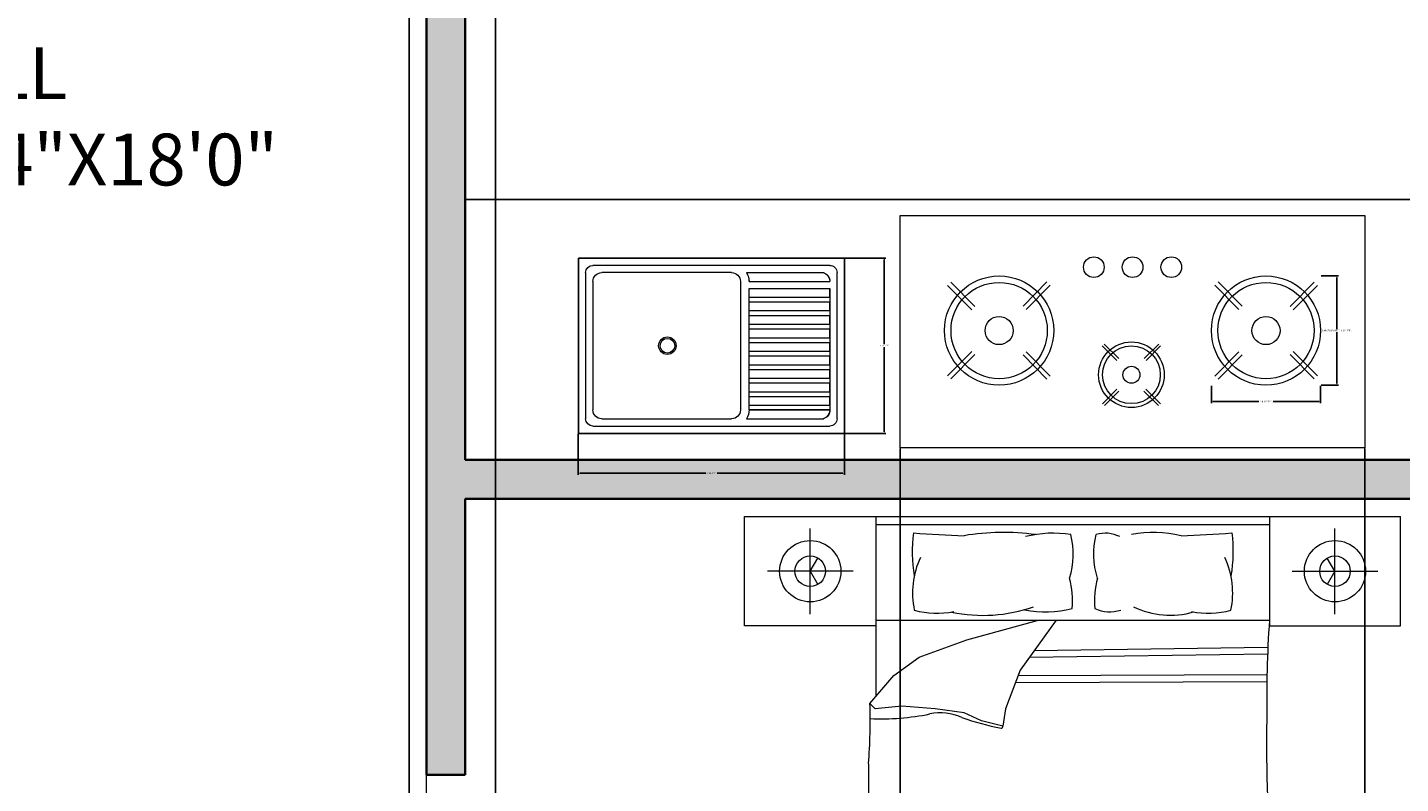
# Model space of a CAD drawing. Units: inches. Extents: x -5 to 366, y -496 to 54.
# Tile 6 of 10: x 121 to 280, y -293 to -205. Entities that reach past the tile are written whole.
import ezdxf

# ---------------------------------------------------------------- set-up
doc = ezdxf.new("R2010")
doc.units = ezdxf.units.IN
doc.header["$MEASUREMENT"] = 0
for name, color, linetype, lineweight in [('A-ANNO-DIMS', 2, 'Continuous', 18), ('A-AREA-IDEN', 7, 'Continuous', 25), ('A-DOOR', 3, 'Continuous', 18), ('A-EQPM', 9, 'Continuous', 18), ('A-FLOR-CASE', 7, 'Continuous', 25), ('A-FLOR-FIXT', 9, 'Continuous', 18), ('A-FURN', 8, 'Continuous', 18), ('A-WALL', 7, 'Continuous', 35), ('A-WALL-PATT', 252, 'Continuous', 13)]:
    doc.layers.add(name, color=color, linetype=linetype, lineweight=lineweight)
doc.styles.get("Standard").update_dxf_attribs({"font": 'arial.ttf'})
doc.dimstyles.get("Standard").update_dxf_attribs({"dimtxt": 0.18, "dimasz": 0.18, "dimexe": 0.18, "dimexo": 0.0625, "dimgap": 0.09, "dimtad": 0, "dimtih": 1, "dimtoh": 1, "dimdec": 0, "dimzin": 0, "dimdsep": 46, "dimlunit": 3, "dimtxsty": 'Standard', "dimcen": 0.09, "dimadec": 0, "dimazin": 0, "dimtfac": 1, "dimtdec": 0, "dimtofl": 0, "dimtmove": 0, "dimatfit": 3, "dimfxl": 1, "dimtolj": 1, "dimtzin": 0, "dimarcsym": 0})

# ---------------------------------------------------------------- blocks, each defined once
blk = doc.blocks.new('М12 540х820')
for p, q in [((0, 540), (-820, 540)), ((-820, 540), (-820, 0)), ((-45, 517.5), (-775, 517.5)), ((0, 0), (0, 540)), ((-797.5, 495), (-797.5, 45)), ((-775, 468), (-775, 72)), ((-347.5, 495), (-748, 495)), ((-320.5, 468), (-320.5, 72)), ((-301.7, 495), (-64.8, 495)), ((-293.7, 468), (-293.7, 472.5)), ((-293.7, 468), (-45, 468)), ((-45, 469.5), (-45, 468)), ((-22.5, 45), (-22.5, 495)), ((-293.7, 446.6), (-45, 446.6)), ((-293.7, 419.6), (-293.7, 446.6)), ((-45, 419.6), (-45, 446.6)), ((-293.7, 419.6), (-45, 419.6)), ((-293.7, 405), (-45, 405)), ((-293.7, 378), (-293.7, 405)), ((-45, 378), (-45, 405)), ((-293.7, 378), (-45, 378)), ((-293.7, 336.4), (-293.7, 363.4)), ((-293.7, 363.4), (-45, 363.4)), ((-45, 336.4), (-45, 363.4)), ((-293.7, 336.4), (-45, 336.4)), ((-293.7, 294.7), (-293.7, 321.7)), ((-293.7, 321.7), (-45, 321.7)), ((-45, 294.7), (-45, 321.7)), ((-293.7, 294.7), (-45, 294.7)), ((-293.7, 253.1), (-293.7, 280.1)), ((-293.7, 280.1), (-45, 280.1)), ((-45, 253.1), (-45, 280.1)), ((-293.7, 253.1), (-45, 253.1)), ((-293.7, 211.5), (-293.7, 238.5)), ((-293.7, 238.5), (-45, 238.5)), ((-45, 211.5), (-45, 238.5)), ((-293.7, 211.5), (-45, 211.5)), ((-293.7, 169.9), (-293.7, 196.9)), ((-293.7, 196.9), (-45, 196.9)), ((-293.7, 169.9), (-45, 169.9)), ((-45, 169.9), (-45, 196.9)), ((-293.7, 128.2), (-293.7, 155.2)), ((-293.7, 155.2), (-45, 155.2)), ((-293.7, 128.2), (-45, 128.2)), ((-45, 128.2), (-45, 155.2)), ((-293.7, 113.6), (-45, 113.6)), ((-293.7, 86.6), (-293.7, 113.6)), ((-293.7, 86.6), (-45, 86.6)), ((-45, 86.6), (-45, 113.6)), ((-748, 45), (-347.5, 45)), ((-301.7, 45), (-64.8, 45)), ((-293.7, 72), (-45, 72)), ((-45, 70.5), (-45, 72)), ((-820, 0), (0, 0)), ((-775, 22.5), (-45, 22.5))]:
    blk.add_line(p, q)
at = {"ltscale": 0.06}
for p, q in [((-820, 0), (-820, 540)), ((-820, 540), (0, 540)), ((0, 540), (0, 536.9)), ((0, 536.9), (0, 0)), ((-293.7, 446.6), (-45, 446.6)), ((-293.7, 405), (-293.7, 446.6)), ((-45, 446.6), (-45, 419.6)), ((-293.7, 363.4), (-293.7, 405)), ((-45, 419.6), (-45, 378)), ((-293.7, 321.7), (-293.7, 363.4)), ((-45, 378), (-45, 336.4)), ((-293.7, 280.1), (-293.7, 321.7)), ((-45, 336.4), (-45, 294.7)), ((-293.7, 238.5), (-293.7, 280.1)), ((-45, 294.7), (-45, 253.1)), ((-293.7, 196.9), (-293.7, 238.5)), ((-45, 253.1), (-45, 211.5)), ((-293.7, 155.2), (-293.7, 196.9)), ((-45, 211.5), (-45, 169.9)), ((-45, 169.9), (-45, 128.2)), ((-293.7, 113.6), (-293.7, 155.2)), ((-45, 128.2), (-45, 86.6)), ((-293.7, 72), (-293.7, 113.6)), ((-45, 86.6), (-45, 72)), ((-45, 72), (-293.7, 72)), ((0, 0), (-820, 0))]:
    blk.add_line(p, q, dxfattribs=at)
at = {"extrusion": (0, 0, -1)}
for centre, major_axis, start_param, end_param in [((-775, 495), (-15.9, 15.9), -0.785398, 0.785398), ((-775, 495), (-15.9, 15.9), -0.785398, 0.785398), ((-45, 495), (-15.9, -15.9), 2.356194, 3.926991), ((-45, 495), (-15.9, -15.9), 2.356194, 3.926991), ((-748, 468), (-19.1, -19.1), 0.785398, 2.356194), ((-748, 468), (-19.1, -19.1), 0.785398, 2.356194), ((-347.5, 468), (-19.1, 19.1), 0.785398, 2.356194), ((-347.5, 468), (-19.1, 19.1), 0.785398, 2.356194), ((-343.2, 468), (-35, 35), 1.779263, 2.356194), ((-343.2, 468), (-35, 35), 1.779263, 2.356192), ((-343.2, 468), (-35, 35), 2.356192, 2.356194), ((-72.3, 468.8), (-19.3, 19.3), 1.0328, 2.38382), ((-72.3, 468.8), (-19.3, 19.3), 1.0328, 1.064673), ((-72.3, 468.8), (-19.3, 19.3), 1.064673, 2.328569), ((-72.3, 468.8), (-19.3, 19.3), 2.328569, 2.38382), ((-545.5, 270), (-19.1, -19.1), 3.926991, 10.210176), ((-545.5, 270), (-19.1, -19.1), 3.926991, 10.210176), ((-545.5, 270), (-15.9, -15.9), 3.926991, 10.210176), ((-545.5, 270), (-15.9, -15.9), 3.926991, 10.210176), ((-775, 45), (-15.9, -15.9), 5.497787, 7.068583), ((-775, 45), (-15.9, -15.9), 5.497787, 7.068583), ((-748, 72), (-19.1, 19.1), 3.926991, 5.497787), ((-748, 72), (-19.1, 19.1), 3.926991, 5.497787), ((-347.5, 72), (-19.1, -19.1), 3.926991, 5.497787), ((-347.5, 72), (-19.1, -19.1), 3.926991, 5.497787), ((-343.2, 72), (-35, -35), 3.926991, 4.503922), ((-343.2, 72), (-35, -35), 3.926991, 4.503922), ((-72.3, 71.2), (-19.3, -19.3), 3.899365, 5.250385), ((-72.3, 71.2), (-19.3, -19.3), 5.218512, 5.250385), ((-72.3, 71.2), (-19.3, -19.3), 3.954617, 5.218512), ((-72.3, 71.2), (-19.3, -19.3), 3.899365, 3.954617), ((-45, 45), (-15.9, 15.9), 2.356194, 3.926991), ((-45, 45), (-15.9, 15.9), 2.356194, 3.926991)]:
    blk.add_ellipse(centre, major_axis=major_axis, ratio=1, start_param=start_param, end_param=end_param, dxfattribs=at)
blk = doc.blocks.new('BED-DOUBLE-WITH-NIGHTSTANDS')
for p, q in [((0, 64.67), (76.05, 64.67)), ((15.21, 64.67), (15.21, 43.8)), ((60.84, 63.7), (15.21, 63.7)), ((7.61, 53.37), (7.61, 63.31)), ((68.45, 53.37), (68.45, 63.31)), ((12.58, 58.34), (2.64, 58.34)), ((63.48, 58.34), (73.42, 58.34)), ((15.21, 52.66), (60.84, 52.66)), ((25.78, 50.4), (34.07, 52.66)), ((36.11, 52.66), (31.94, 46.86)), ((20.23, 48.39), (25.78, 50.4)), ((60.64, 49.5), (33.56, 49.12)), ((17.3, 46.24), (20.23, 48.39)), ((60.61, 48.72), (33, 48.33)), ((14.53, 43.01), (17.3, 46.24)), ((31.94, 46.86), (30.24, 42.39)), ((60.57, 46.32), (31.69, 46.21)), ((60.58, 45.54), (31.39, 45.42)), ((15.15, 42.39), (14.53, 43.01)), ((18.23, 42.7), (15.15, 42.39)), ((22.08, 42.39), (18.23, 42.7)), ((25.47, 41.93), (22.08, 42.39)), ((27.47, 41.01), (25.47, 41.93)), ((30.24, 42.39), (29.94, 40.39)), ((29.94, 40.39), (27.47, 41.01)), ((10.04, 27.39), (14.34, 27.39)), ((10.04, 0), (10.04, 27.39)), ((61.27, 27.39), (65.49, 27.39)), ((65.49, 27.39), (65.49, 0)), ((14.34, 26.51), (10.92, 26.51)), ((10.92, 26.51), (10.92, 0.88)), ((64.6, 26.51), (61.25, 26.51)), ((64.6, 0.88), (64.6, 26.51)), ((61.19, 22.65), (14.34, 22.65)), ((61.26, 21.7), (14.34, 21.7)), ((53.47, 14.23), (22.59, 14.23)), ((18.42, 8.59), (18.25, 9.45)), ((23.73, 8.59), (23.9, 9.45)), ((51.79, 8.59), (51.63, 9.45)), ((57.11, 8.59), (57.28, 9.45)), ((10.92, 0.88), (64.6, 0.88)), ((65.49, 0), (10.04, 0))]:
    blk.add_line(p, q)
for points in [[(15.21, 52), (0, 52), (0, 64.67)], [(60.84, 64.67), (60.84, 52), (76.05, 52), (76.05, 64.67)], [(7.61, 58.34), (8.49, 59.87)], [(68.45, 58.34), (67.56, 59.87)], [(7.61, 58.34), (8.49, 56.8)], [(68.45, 58.34), (67.56, 56.8)]]:
    blk.add_lwpolyline(points)
for points in [[(19.58, 62.78, 0.074897), (19.67, 57.81, -0.472817)], [(37.67, 57.53, 0.14099), (37.82, 62.6, 0.235245)], [(40.92, 57.53, -0.14099), (40.77, 62.6, -0.235245)], [(56.48, 62.78, -0.074897), (56.38, 57.81, 0.472817)], [(14.37, 36.04, 0.001242), (14.34, 21.61, -0.127202), (12.81, 14.42)], [(61.17, 23.25, 0.056112), (61.72, 19.07, 0.095341), (62.79, 15.03)]]:
    blk.add_lwpolyline(points, format="xyb")
for centre, radius in [((7.61, 58.34), 3.55), ((68.45, 58.34), 3.55), ((7.61, 58.34), 1.77), ((68.45, 58.34), 1.77), ((22.81, 5.83), 0.194), ((52.72, 5.83), 0.194), ((21.54, 3.79), 0.194), ((53.98, 3.79), 0.194)]:
    blk.add_circle(centre, radius)
for centre, radius, start, end in [((61.5, 786.54), 724.98, 266.68521, 267.14978), ((30, 35.26), 27.58, 82.2196, 99.497), ((35.83, 49.2), 13.55, 81.5249, 103.96), ((41.81, 58.99), 3.76, 63.3437, 106.1026), ((47.45, 49.47), 13.37, 76.3427, 101.1841), ((14.56, 786.54), 724.98, 272.85022, 273.31479), ((29.27, 55.82), 9.8, 155.1316, 191.7583), ((46.79, 55.82), 9.8, 348.2417, 24.8684), ((28.71, 54.99), 9.32, 354.0129, 15.8293), ((49.88, 54.99), 9.32, 164.1707, 185.9871), ((27.66, 70.91), 17.68, 258.0397, 289.2615), ((49.36, 62.92), 9.68, 243.8761, 286.1746), ((22.29, 63.67), 10.19, 255.1039, 281.0369), ((34.82, 67.05), 13.41, 259.8617, 283.6238), ((42.32, 57.67), 4.03, 245.0183, 288.5407), ((53.76, 63.67), 10.19, 258.9631, 284.8961), ((197.18, 43.36), 136.65, 176.1, 180.9282), ((-55.2, 41.12), 69.76, 355.8294, 1.553), ((15.83, 69.94), 28.7, 267.4519, 281.3392), ((22.69, 35.73), 6.19, 66.2616, 101.3392), ((35.22, 69.13), 29.49, 250.1194, 259.3383), ((29.76, 40.33), 0.184, 268.8623, 19.7536), ((238.78, 38.39), 178.26, 179.1145, 184.8735), ((13.51, 14.47), 0.702, 183.98, 297.3412), ((62.21, 14.65), 0.693, 246.5219, 33.8264), ((21.68, -64.93), 79.17, 89.3433, 95.6887), ((16.57, 11.64), 1.28, 84.4856, 181.0538), ((13.22, 8.88), 5.76, 33.6671, 63.2997), ((16.17, 10.69), 2.29, 355.2933, 76.921), ((20.93, 12.3), 2.93, 145.785, 184.7304), ((15.33, 13.67), 3.15, 328.8218, 9.1554), ((19.23, 13.39), 0.916, 120.0293, 142.325), ((17.77, 12.85), 2.42, 289.2822, 29.1751), ((17.4, 12.41), 2.19, 7.436, 29.9149), ((18.84, 13.57), 1.14, 311.5653, 23.8354), ((19.23, 13.39), 0.916, 44.4517, 63.558), ((24.38, 12.85), 2.42, 150.8249, 250.7178), ((23.31, 13.57), 1.14, 156.1646, 228.4347), ((22.92, 13.39), 0.916, 113.229, 135.5483), ((24.75, 12.41), 2.19, 150.0851, 172.564), ((22.92, 13.39), 0.916, 37.675, 66.7144), ((21.22, 12.3), 2.93, 355.2696, 34.215), ((26.82, 13.67), 3.15, 169.7133, 211.1782), ((25.97, 10.69), 2.29, 103.079, 184.7067), ((28.93, 8.88), 5.76, 111.4941, 146.3329), ((25.58, 11.64), 1.28, 358.9462, 95.5144), ((49.95, 11.64), 1.28, 84.4856, 181.0538), ((46.59, 8.88), 5.76, 33.6671, 68.5059), ((49.55, 10.69), 2.29, 355.2933, 76.921), ((54.31, 12.3), 2.93, 145.785, 184.7304), ((48.7, 13.67), 3.15, 328.8218, 10.2867), ((52.61, 13.39), 0.916, 113.2856, 142.325), ((51.15, 12.85), 2.42, 289.2822, 29.1751), ((50.78, 12.41), 2.19, 7.436, 29.9149), ((52.61, 13.39), 0.916, 44.4517, 66.7144), ((52.22, 13.57), 1.14, 311.5653, 23.8354), ((55.8, -59.74), 74, 85.2402, 91.8035), ((57.76, 12.85), 2.42, 150.8249, 250.7178), ((56.68, 13.57), 1.14, 156.1646, 228.4347), ((56.3, 13.39), 0.916, 106.6343, 135.5483), ((58.13, 12.41), 2.19, 150.0851, 172.564), ((56.3, 13.39), 0.916, 37.675, 72.5814), ((54.6, 12.3), 2.93, 355.2696, 34.215), ((60.2, 13.67), 3.15, 169.249, 211.1782), ((59.35, 10.69), 2.29, 103.079, 184.7067), ((62.31, 8.88), 5.76, 113.6453, 146.3329), ((58.96, 11.64), 1.28, 358.9462, 95.5144), ((17.09, 11.46), 1.82, 174.9449, 262.8857), ((17.81, 12.15), 1.76, 201.5819, 291.4221), ((17.47, 10.23), 1.89, 299.9085, 73.1337), ((18.67, 11.02), 0.472, 257.3041, 15.1471), ((20.63, 11.55), 1.56, 131.5653, 195.1471), ((21.52, 11.55), 1.56, 344.8529, 48.4347), ((24.67, 10.23), 1.89, 106.8663, 240.0915), ((23.48, 11.02), 0.472, 164.8529, 282.6959), ((24.34, 12.15), 1.76, 248.5779, 338.4181), ((25.05, 11.46), 1.82, 277.1143, 5.0551), ((50.47, 11.46), 1.82, 174.9449, 262.8857), ((51.19, 12.15), 1.76, 201.5819, 291.4221), ((50.85, 10.23), 1.89, 299.9085, 73.1337), ((52.05, 11.02), 0.472, 257.3041, 15.1471), ((54.01, 11.55), 1.56, 131.5653, 195.1471), ((54.89, 11.55), 1.56, 344.8529, 48.4347), ((58.05, 10.23), 1.89, 106.8663, 240.0915), ((56.86, 11.02), 0.472, 164.8529, 282.6959), ((57.72, 12.15), 1.76, 248.5779, 338.4181), ((58.43, 11.46), 1.82, 277.1143, 5.0551), ((16.68, 8.53), 1.14, 80.264, 250.8688), ((14.41, 11.04), 3.59, 301.2614, 341.7045), ((16.78, 11.86), 2.21, 272.3591, 324.0401), ((14.38, 10.75), 4.08, 326.2883, 356.5076), ((20.93, 12.3), 2.93, 212.7011, 216.3445), ((21.29, 10.31), 0.147, 102.7051, 280.4384), ((21.28, 10.4), 0.238, 280.4384, 100.4136), ((21.22, 12.3), 2.93, 323.6555, 327.2989), ((25.37, 11.86), 2.21, 215.9599, 267.6409), ((27.77, 10.75), 4.08, 183.4924, 213.7117), ((27.73, 11.04), 3.59, 198.2955, 238.7386), ((25.47, 8.53), 1.14, 289.1312, 99.736), ((38.64, 9.21), 0.823, 63.0274, 163.8037), ((37.8, 11.14), 1.7, 271.4585, 315.3727), ((38.49, 8.01), 1.57, 45.5411, 114.3101), ((39.57, 8.01), 1.57, 65.6899, 134.4589), ((39.42, 9.21), 0.823, 16.1963, 116.9726), ((40.26, 11.14), 1.7, 224.6273, 268.5415), ((50.06, 8.53), 1.14, 80.264, 250.8688), ((47.79, 11.04), 3.59, 301.2614, 341.7045), ((50.16, 11.86), 2.21, 272.3591, 324.0401), ((47.76, 10.75), 4.08, 326.2883, 356.5076), ((54.31, 12.3), 2.93, 212.7011, 216.3445), ((54.25, 10.4), 0.238, 79.5864, 259.5616), ((54.23, 10.31), 0.147, 259.5616, 77.2949), ((54.6, 12.3), 2.93, 323.6555, 327.2989), ((58.75, 11.86), 2.21, 215.9599, 267.6409), ((61.15, 10.75), 4.08, 183.4924, 213.7117), ((61.11, 11.04), 3.59, 198.2955, 238.7386), ((58.85, 8.53), 1.14, 289.1312, 99.736), ((16.44, 7.29), 0.7, 63.9755, 143.2681), ((16.4, 8.87), 1.43, 265.969, 344.3045), ((17.94, 6.98), 1.52, 96.1662, 141.5825), ((20.45, 8.04), 0.399, 101.3256, 154.4621), ((19.88, 9.4), 1.2, 280.2588, 300.656), ((20.15, 10.36), 2.14, 268.3264, 277.1302), ((26.56, 6.48), 6.3, 163.5842, 183.8277), ((19.62, 9.39), 1.22, 308.2101, 316.3071), ((20.37, 8.59), 0.365, 278.3432, 4.2869), ((20.17, 8.91), 0.637, 300.656, 332.6341), ((20.64, 8.49), 0.155, 55.7657, 157.4417), ((26.56, 6.48), 6.3, 153.0032, 159.8941), ((20.89, 8.63), 0.155, 84.3784, 186.0543), ((20.74, 9.25), 0.637, 269.1859, 301.164), ((20.93, 8.93), 0.365, 237.5332, 323.4768), ((20.57, 9.97), 1.22, 285.5129, 293.6099), ((21.37, 8.59), 0.399, 87.3579, 140.4944), ((20.45, 9.74), 1.2, 301.164, 321.5612), ((19.47, 9.95), 2.14, 324.6898, 333.4936), ((24.21, 6.98), 1.52, 38.4175, 83.8338), ((25.74, 8.87), 1.43, 195.6955, 274.031), ((25.71, 7.29), 0.7, 36.7319, 116.0245), ((38.62, -0.46), 9.93, 94.4623, 172.255), ((38.66, 8.7), 1.1, 137.7873, 219.1145), ((37.41, 8.74), 0.829, 298.5391, 58.3627), ((39.93, 16.07), 6.95, 252.593, 267.2582), ((38.66, 9.41), 0.812, 177.7585, 283.852), ((40.22, 10.26), 2.51, 198.9159, 238.011), ((38.14, 16.07), 6.95, 272.7418, 287.407), ((38.83, 8.73), 0.107, 283.852, 219.9245), ((38.96, 8.23), 0.123, 238.011, 71.5592), ((38.98, 8.29), 0.0599, 71.5592, 188.0167), ((39.1, 8.23), 0.123, 108.4408, 301.989), ((39.08, 8.29), 0.0599, 351.9833, 108.4408), ((39.22, 8.77), 0.0647, 320.1909, 256.0209), ((37.84, 10.26), 2.51, 301.989, 341.0841), ((39.4, 9.41), 0.812, 256.148, 2.2415), ((40.65, 8.74), 0.829, 121.6373, 241.4609), ((39.4, 8.7), 1.1, 320.8855, 42.2127), ((39.12, 1.83), 7.69, 352.8636, 81.8197), ((49.82, 7.29), 0.7, 63.9755, 143.2681), ((49.78, 8.87), 1.43, 265.969, 344.3045), ((51.32, 6.98), 1.52, 96.1662, 141.5825), ((55.08, 9.74), 1.2, 218.4388, 238.836), ((54.15, 8.59), 0.399, 39.5056, 92.6421), ((56.06, 9.95), 2.14, 206.5064, 215.3102), ((54.6, 8.93), 0.365, 216.5232, 302.4668), ((54.95, 9.97), 1.22, 246.3901, 254.4871), ((54.79, 9.25), 0.637, 238.836, 270.8141), ((48.96, 6.48), 6.3, 20.1059, 26.9968), ((54.64, 8.63), 0.155, 353.9457, 95.6216), ((54.88, 8.49), 0.155, 22.5583, 124.2343), ((55.16, 8.59), 0.365, 175.7131, 261.6568), ((55.36, 8.91), 0.637, 207.3659, 239.344), ((48.96, 6.48), 6.3, 356.1723, 16.4158), ((55.91, 9.39), 1.22, 223.6929, 231.7899), ((55.65, 9.4), 1.2, 239.344, 259.7412), ((55.37, 10.36), 2.14, 262.8698, 271.6736), ((55.07, 8.04), 0.399, 25.5379, 78.6744), ((59.12, 8.87), 1.43, 195.6955, 274.031), ((57.59, 6.98), 1.52, 38.4175, 83.8338), ((59.08, 7.29), 0.7, 36.7319, 116.0245), ((20.52, -1.44), 9.93, 124.3865, 158.5908), ((15.99, 6.52), 1.1, 167.7115, 249.0387), ((15.71, 6.95), 0.823, 92.9516, 193.728), ((14.03, 8.2), 1.7, 301.3827, 345.2969), ((16.18, 5.84), 1.57, 75.4653, 144.2343), ((13.4, 13.54), 6.95, 282.5173, 297.1824), ((14.89, 5.93), 0.829, 328.4633, 88.2869), ((16.56, 8.65), 2.51, 228.8402, 267.9352), ((15.63, 7.13), 0.812, 207.6827, 313.7762), ((16.12, 6.62), 0.107, 313.7762, 249.7183), ((16.46, 6.32), 0.0599, 101.4834, 217.9409), ((16.48, 6.26), 0.123, 267.9352, 101.4834), ((19.32, 7.28), 0.323, 101.5637, 142.6358), ((19.06, 6.98), 0.194, 273.2768, 86.7232), ((19.32, 6.63), 0.32, 217.7621, 259.0403), ((19.28, 7.17), 0.185, 91.1081, 181.8675), ((19.66, 7.05), 0.588, 203.4276, 227.6104), ((19.48, 6.8), 0.4, 80.3487, 133.6538), ((19.41, 7.13), 0.317, 229.7889, 317.6792), ((19.06, 7.54), 0.466, 288.7263, 352.5032), ((19.05, 6.46), 0.45, 355.053, 68.3618), ((19.4, 6.38), 0.634, 83.0852, 105.7171), ((19.38, 7.52), 0.15, 345.2356, 144.9248), ((19.35, 6.43), 0.149, 232.4737, 355.053), ((15.01, 1.12), 7.22, 43.1541, 52.0459), ((19.52, 7.03), 0.167, 317.6792, 80.3487), ((21.33, 6.12), 0.883, 304.5369, 16.3699), ((22.55, 5.87), 0.625, 127.3105, 187.9252), ((21.7, 5.94), 0.641, 355.0106, 41.658), ((23.08, 6.13), 0.323, 101.5637, 176.365), ((23.14, 6.36), 0.15, 345.2356, 144.9248), ((25.67, 6.26), 0.123, 78.5166, 272.0648), ((25.96, 5.84), 1.57, 35.7657, 104.5347), ((28.74, 13.54), 6.95, 242.8176, 257.4827), ((25.58, 8.65), 2.51, 272.0648, 311.1598), ((25.68, 6.32), 0.0599, 322.0591, 78.5166), ((26.52, 7.13), 0.812, 226.2238, 332.3173), ((26.04, 6.66), 0.0647, 290.2667, 226.2271), ((27.26, 5.93), 0.829, 91.7131, 211.5367), ((26.44, 6.95), 0.823, 346.272, 87.0484), ((28.12, 8.2), 1.7, 194.7031, 238.6173), ((26.16, 6.52), 1.1, 290.9613, 12.2885), ((21.63, -1.44), 9.93, 21.4092, 55.6135), ((53.9, -1.44), 9.93, 124.3865, 158.5908), ((49.36, 6.52), 1.1, 167.7115, 249.0387), ((49.09, 6.95), 0.823, 92.9516, 193.728), ((47.41, 8.2), 1.7, 301.3827, 345.2969), ((49.56, 5.84), 1.57, 75.4653, 144.2343), ((46.78, 13.54), 6.95, 282.5173, 297.1824), ((49.01, 7.13), 0.812, 207.6827, 313.7762), ((49.94, 8.65), 2.51, 228.8402, 267.9352), ((48.26, 5.93), 0.829, 328.4633, 88.2869), ((49.5, 6.62), 0.107, 313.7762, 249.7183), ((49.84, 6.32), 0.0599, 101.4834, 217.9409), ((49.86, 6.26), 0.123, 267.9352, 101.4834), ((52.39, 6.36), 0.15, 35.0752, 194.7644), ((52.45, 6.13), 0.323, 3.635, 78.4363), ((53.83, 5.94), 0.641, 138.342, 184.9894), ((54.2, 6.12), 0.883, 163.6301, 235.4631), ((52.97, 5.87), 0.625, 352.0748, 52.6895), ((60.52, 1.12), 7.22, 127.9541, 136.8459), ((56.01, 7.03), 0.167, 99.6513, 222.3208), ((56.12, 7.13), 0.317, 222.3208, 310.2111), ((56.05, 6.8), 0.4, 46.3462, 99.6513), ((56.15, 7.52), 0.15, 35.0752, 194.7644), ((56.46, 7.54), 0.466, 187.4968, 251.2737), ((56.48, 6.46), 0.45, 111.6382, 184.947), ((56.18, 6.43), 0.149, 184.947, 307.5263), ((56.12, 6.38), 0.634, 74.2829, 96.9148), ((56.25, 7.17), 0.185, 358.1325, 88.8919), ((55.86, 7.05), 0.588, 312.3896, 336.5724), ((56.2, 7.28), 0.323, 37.3642, 78.4363), ((56.21, 6.63), 0.32, 280.9597, 322.2379), ((56.47, 6.98), 0.194, 93.2768, 266.7232), ((59.05, 6.26), 0.123, 78.5166, 272.0648), ((59.34, 5.84), 1.57, 35.7657, 104.5347), ((62.12, 13.54), 6.95, 242.8176, 257.4827), ((58.96, 8.65), 2.51, 272.0648, 311.1598), ((59.06, 6.32), 0.0599, 322.0591, 78.5166), ((59.9, 7.13), 0.812, 226.2238, 332.3173), ((59.42, 6.66), 0.0647, 290.2667, 226.2271), ((60.64, 5.93), 0.829, 91.7131, 211.5367), ((61.5, 8.2), 1.7, 194.7031, 238.6173), ((59.82, 6.95), 0.823, 346.272, 87.0484), ((59.54, 6.52), 1.1, 290.9613, 12.2885), ((55.01, -1.44), 9.93, 21.4092, 55.6135), ((3.53, -0.46), 9.93, 7.745, 41.8856), ((20, 5.48), 0.399, 101.3256, 154.4621), ((19.42, 6.84), 1.2, 280.2588, 300.656), ((19.7, 7.8), 2.14, 268.3264, 277.1302), ((19.17, 6.83), 1.22, 308.2101, 316.3071), ((20.13, 4.78), 0.216, 146.8636, 236.9021), ((23.18, 9.55), 5.66, 235.1882, 238.8844), ((20.5, 5.1), 0.585, 199.4799, 267.6828), ((19.91, 6.03), 0.365, 278.3432, 4.2869), ((19.71, 6.35), 0.637, 300.656, 332.6341), ((20.19, 5.93), 0.155, 55.7657, 157.4417), ((23.43, 6.32), 3.16, 184.756, 209.2041), ((27.97, 13.04), 10.39, 222.2412, 232.1744), ((20.65, 4.61), 0.169, 311.8703, 134.2646), ((21.14, 5.38), 0.883, 247.2305, 319.0635), ((23.75, 2.13), 3.79, 120.544, 139.818), ((21.59, 4.21), 0.625, 70.0041, 130.6188), ((21.19, 4.97), 0.641, 297.7043, 344.3516), ((21.8, 5.92), 0.537, 272.8499, 356.1226), ((21.42, 5.72), 0.52, 321.7607, 7.9252), ((21.53, 4.97), 0.52, 8.7227, 54.8872), ((21.56, 4.55), 0.883, 0.278, 72.111), ((21.95, 4.88), 0.537, 20.5253, 88.5375), ((22.66, 5.14), 0.625, 188.7227, 249.3375), ((22.4, 5.47), 0.192, 148.0499, 225.6268), ((23.75, 2.13), 3.79, 113.0501, 113.8477), ((22.76, 5.25), 0.611, 104.7558, 148.0499), ((22.42, 5.69), 0.382, 247.4086, 351.4386), ((22.6, 6.1), 0.264, 126.1046, 271.4281), ((22.57, 6.17), 0.19, 353.7526, 131.7054), ((21.86, 4.83), 0.641, 334.9899, 21.6373), ((22.52, 5.67), 0.128, 262.906, 7.132), ((22.39, 5.95), 0.267, 0.0645, 61.1507), ((22.45, 6.18), 0.305, 311.8413, 355.7877), ((23.07, 5.47), 0.32, 151.2196, 259.0403), ((23.04, 6.02), 0.185, 91.1081, 181.8675), ((23.42, 5.9), 0.588, 203.4276, 227.6104), ((23.23, 5.64), 0.4, 80.3487, 133.6538), ((23.16, 5.98), 0.317, 229.7889, 317.6792), ((22.82, 6.39), 0.466, 288.7263, 352.5032), ((22.8, 5.3), 0.45, 355.053, 68.3618), ((23.16, 5.23), 0.634, 83.0852, 105.7171), ((23.1, 5.28), 0.149, 232.4737, 355.053), ((23.27, 5.87), 0.167, 317.6792, 80.3487), ((23.75, 2.13), 3.79, 87.1071, 94.7585), ((51.78, 2.13), 3.79, 85.2415, 92.8929), ((52.25, 5.87), 0.167, 99.6513, 222.3208), ((52.37, 5.98), 0.317, 222.3208, 310.2111), ((52.29, 5.64), 0.4, 46.3462, 99.6513), ((52.71, 6.39), 0.466, 187.4968, 251.2737), ((52.72, 5.3), 0.45, 111.6382, 184.947), ((52.42, 5.28), 0.149, 184.947, 307.5263), ((52.37, 5.23), 0.634, 74.2829, 96.9148), ((52.49, 6.02), 0.185, 358.1325, 88.8919), ((52.11, 5.9), 0.588, 312.3896, 336.5724), ((52.45, 5.47), 0.32, 280.9597, 28.7804), ((53.11, 5.69), 0.382, 188.5614, 292.5914), ((52.96, 6.17), 0.19, 48.2946, 186.2474), ((53.07, 6.18), 0.305, 184.2123, 228.1587), ((53.14, 5.95), 0.267, 118.8493, 179.9355), ((53, 5.67), 0.128, 172.868, 277.094), ((52.93, 6.1), 0.264, 268.5719, 53.8954), ((52.77, 5.25), 0.611, 31.9501, 75.2442), ((53.67, 4.83), 0.641, 158.3627, 205.0101), ((53.57, 4.88), 0.537, 91.4625, 159.4747), ((53.97, 4.55), 0.883, 107.889, 179.722), ((52.87, 5.14), 0.625, 290.6625, 351.2773), ((53.73, 5.92), 0.537, 183.8774, 267.1501), ((51.78, 2.13), 3.79, 66.1523, 66.9499), ((53.12, 5.47), 0.192, 314.3732, 31.9501), ((54, 4.97), 0.52, 125.1128, 171.2773), ((54.11, 5.72), 0.52, 172.0748, 218.2393), ((51.78, 2.13), 3.79, 40.182, 59.456), ((53.93, 4.21), 0.625, 49.3812, 109.9959), ((54.39, 5.38), 0.883, 220.9365, 292.7695), ((54.34, 4.97), 0.641, 195.6484, 242.2957), ((47.55, 13.04), 10.39, 307.8256, 317.7588), ((54.88, 4.61), 0.169, 45.7354, 228.1297), ((52.1, 6.32), 3.16, 330.7959, 355.244), ((55.02, 5.1), 0.585, 272.3172, 340.5201), ((55.33, 5.93), 0.155, 22.5583, 124.2343), ((55.61, 6.03), 0.365, 175.7131, 261.6568), ((55.81, 6.35), 0.637, 207.3659, 239.344), ((52.34, 9.55), 5.66, 301.1156, 304.8118), ((56.36, 6.83), 1.22, 223.6929, 231.7899), ((56.1, 6.84), 1.2, 239.344, 259.7412), ((55.39, 4.78), 0.216, 303.0979, 33.1364), ((55.82, 7.8), 2.14, 262.8698, 271.6736), ((55.53, 5.48), 0.399, 25.5379, 78.6744), ((72, -0.46), 9.93, 138.1144, 172.255), ((20.44, 4.87), 0.504, 212.8155, 277.3992), ((20.15, 4.54), 0.585, 266.9701, 338.2913), ((17.06, 8.72), 5.66, 302.6784, 306.3746), ((20.29, 4.07), 0.216, 214.3538, 304.3923), ((20.37, 4.89), 0.224, 238.8844, 314.2646), ((20.33, 4.39), 0.504, 280.3057, 17.1958), ((20.28, 4.34), 0.224, 306.3746, 21.7548), ((20.65, 4.49), 0.169, 19.3605, 201.7548), ((23.82, 3.07), 3.37, 153.7819, 158.2913), ((20.85, 5.08), 0.52, 264.4544, 310.6188), ((23.43, 6.32), 3.16, 214.0033, 222.4917), ((21.23, 4.87), 0.537, 218.3208, 298.8162), ((21.14, 3.43), 0.192, 148.0499, 225.6268), ((21.49, 3.21), 0.611, 104.7558, 148.0499), ((21.15, 3.64), 0.382, 247.4086, 351.4386), ((21.33, 4.06), 0.264, 126.1046, 271.4281), ((21.3, 4.13), 0.19, 353.7526, 131.7054), ((21.26, 3.63), 0.128, 262.906, 7.132), ((21.12, 3.91), 0.267, 0.0645, 61.1507), ((21.18, 4.13), 0.305, 311.8413, 355.7877), ((21.81, 4.09), 0.323, 101.5637, 176.365), ((21.81, 3.43), 0.32, 151.2196, 259.0403), ((21.77, 3.98), 0.185, 91.1081, 181.8675), ((22.15, 3.86), 0.588, 203.4276, 227.6104), ((21.97, 3.6), 0.4, 80.3487, 133.6538), ((21.89, 3.93), 0.317, 229.7889, 317.6792), ((21.55, 4.35), 0.466, 288.7263, 352.5032), ((21.54, 3.26), 0.45, 355.053, 68.3618), ((21.89, 3.19), 0.634, 83.0852, 105.7171), ((21.87, 4.32), 0.15, 345.2356, 144.9248), ((21.84, 3.24), 0.149, 232.4737, 355.053), ((22, 3.83), 0.167, 317.6792, 80.3487), ((37.86, -5.78), 9.93, 94.4623, 117.4146), ((37.9, 3.38), 1.1, 137.7873, 219.1145), ((36.65, 3.42), 0.829, 298.5391, 58.3627), ((37.88, 3.89), 0.823, 63.0274, 163.8037), ((37.04, 5.82), 1.7, 271.4585, 315.3727), ((37.73, 2.69), 1.57, 45.5411, 114.3101), ((39.46, 4.94), 2.51, 198.9159, 238.011), ((39.17, 10.75), 6.95, 252.593, 267.2582), ((37.9, 4.09), 0.812, 177.7585, 283.852), ((38.07, 3.41), 0.107, 283.852, 219.9245), ((40.33, 2.69), 1.57, 65.6899, 134.4589), ((38.9, 10.75), 6.95, 272.7418, 287.407), ((40.18, 3.89), 0.823, 16.1963, 116.9726), ((41.02, 5.82), 1.7, 224.6273, 268.5415), ((39.98, 3.45), 0.0647, 320.1909, 256.0209), ((38.6, 4.94), 2.51, 301.989, 341.0841), ((40.16, 4.09), 0.812, 256.148, 2.2415), ((41.41, 3.42), 0.829, 121.6373, 241.4609), ((40.16, 3.38), 1.1, 320.8855, 42.2127), ((40.2, -5.78), 9.93, 62.5854, 85.5377), ((53.52, 3.83), 0.167, 99.6513, 222.3208), ((53.63, 3.93), 0.317, 222.3208, 310.2111), ((53.56, 3.6), 0.4, 46.3462, 99.6513), ((53.66, 4.32), 0.15, 35.0752, 194.7644), ((53.97, 4.35), 0.466, 187.4968, 251.2737), ((53.99, 3.26), 0.45, 111.6382, 184.947), ((53.69, 3.24), 0.149, 184.947, 307.5263), ((53.64, 3.19), 0.634, 74.2829, 96.9148), ((53.76, 3.98), 0.185, 358.1325, 88.8919), ((53.37, 3.86), 0.588, 312.3896, 336.5724), ((53.72, 4.09), 0.323, 3.635, 78.4363), ((53.72, 3.43), 0.32, 280.9597, 28.7804), ((54.38, 3.64), 0.382, 188.5614, 292.5914), ((54.3, 4.87), 0.537, 241.1838, 321.6792), ((54.23, 4.13), 0.19, 48.2946, 186.2474), ((54.34, 4.13), 0.305, 184.2123, 228.1587), ((54.4, 3.91), 0.267, 118.8493, 179.9355), ((54.27, 3.63), 0.128, 172.868, 277.094), ((54.2, 4.06), 0.264, 268.5719, 53.8954), ((54.03, 3.21), 0.611, 31.9501, 75.2442), ((54.68, 5.08), 0.52, 229.3812, 275.5456), ((52.1, 6.32), 3.16, 317.5083, 325.9967), ((54.39, 3.43), 0.192, 314.3732, 31.9501), ((55.2, 4.39), 0.504, 162.8042, 259.6943), ((54.88, 4.49), 0.169, 338.2452, 160.6395), ((51.7, 3.07), 3.37, 21.7087, 26.2181), ((55.38, 4.54), 0.585, 201.7087, 273.0299), ((55.15, 4.89), 0.224, 225.7354, 301.1156), ((55.09, 4.87), 0.504, 262.6008, 327.1845), ((55.24, 4.34), 0.224, 158.2452, 233.6254), ((58.47, 8.72), 5.66, 233.6254, 237.3216), ((55.23, 4.07), 0.216, 235.6077, 325.6462), ((8.51, -1.79), 4.84, 33.4617, 60.1116), ((6.77, -2.69), 6.03, 36.3036, 46.4814), ((11.22, -0.67), 4.04, 22.5547, 48.9546), ((0.16, 1.5), 13.74, 357.4081, 3.6519), ((30.93, -0.67), 4.04, 131.0454, 157.4453), ((41.99, 1.5), 13.74, 176.3481, 182.5919), ((33.64, -1.79), 4.84, 91.272, 146.5383), ((35.38, -2.69), 6.03, 107.8504, 143.6964), ((38.55, -4.39), 8.97, 124.0123, 144.053), ((38.2, 2.91), 0.123, 238.011, 71.5592), ((38.22, 2.97), 0.0599, 71.5592, 188.0167), ((39.86, 2.91), 0.123, 108.4408, 301.989), ((39.84, 2.97), 0.0599, 351.9833, 108.4408), ((40.11, 2.54), 4.45, 338.117, 6.6195), ((44.19, 1.3), 1.78, 346.3898, 79.0739), ((42.85, 1.54), 2.25, 342.8609, 41.9049), ((33.54, 1.5), 13.74, 357.4081, 3.6519), ((44.6, -0.67), 4.04, 22.5547, 48.9546), ((64.31, -0.67), 4.04, 131.0454, 157.4453), ((75.37, 1.5), 13.74, 176.3481, 182.5919), ((67.02, -1.79), 4.84, 119.8884, 146.5383), ((68.76, -2.69), 6.03, 133.5186, 143.6964), ((35.08, -4.34), 5.46, 73.5431, 107.0202), ((37.25, -7.16), 8.08, 94.3787, 95.6357), ((41.5, -12.69), 14.43, 109.7217, 109.9028), ((42.98, -4.34), 5.46, 72.9798, 106.4569), ((40.82, -7.16), 8.08, 84.3643, 85.6213), ((36.56, -12.69), 14.43, 70.0972, 70.2783)]:
    blk.add_arc(centre, radius, start, end)
blk = doc.blocks.new('COOKTOP-BURNER-LARGE')
for p, q in [((3.19, 8.78), (0.4, 11.6)), ((3.56, 9.14), (0.78, 11.97)), ((9.13, 9.12), (11.93, 11.93)), ((9.5, 8.75), (12.31, 11.56)), ((3.19, 3.88), (0.4, 1.06)), ((3.56, 3.51), (0.78, 0.69)), ((9.13, 3.54), (11.93, 0.73)), ((9.5, 3.91), (12.31, 1.1))]:
    blk.add_line(p, q)
for radius in [6.33, 5.58, 1.63]:
    blk.add_circle((6.33, 6.33), radius)
blk = doc.blocks.new('*D21')
at = {"layer": 'A-ANNO-DIMS', "color": 0, "lineweight": -2, "transparency": 16777216}
for p, q in [((271.18, -234.16), (273.19, -234.16)), ((273.01, -234.34), (273.01, -240.31)), ((273.01, -246.64), (273.01, -240.67)), ((271.18, -246.82), (273.19, -246.82))]:
    blk.add_line(p, q, dxfattribs=at)
at = {"layer": 'A-ANNO-DIMS', "color": 0, "transparency": 16777216}
for points in [[(272.98, -234.34), (273.04, -234.34), (273.01, -234.16)], [(272.98, -246.64), (273.04, -246.64), (273.01, -246.82)]]:
    blk.add_solid(points, dxfattribs=at)
at = {"layer": 'Defpoints', "color": 0, "transparency": 16777216}
for p in [(271.11, -234.16), (273.01, -234.16), (271.11, -246.82)]:
    blk.add_point(p, dxfattribs=at)
at = {"layer": 'A-ANNO-DIMS', "color": 0, "transparency": 16777216, "insert": (273.01, -240.49), "char_height": 0.18, "attachment_point": 5}
blk.add_mtext('\\A1;LARGE BURNER 1\'-0 1/2" TYP.', dxfattribs=at)
blk = doc.blocks.new('*D22')
at = {"layer": 'A-ANNO-DIMS', "color": 0, "lineweight": -2, "transparency": 16777216}
for p, q in [((258.45, -246.88), (258.45, -248.9)), ((271.11, -246.88), (271.11, -248.9)), ((258.63, -248.72), (263.94, -248.72)), ((270.93, -248.72), (265.62, -248.72))]:
    blk.add_line(p, q, dxfattribs=at)
at = {"layer": 'A-ANNO-DIMS', "color": 0, "transparency": 16777216}
for points in [[(258.63, -248.69), (258.63, -248.75), (258.45, -248.72)], [(270.93, -248.69), (270.93, -248.75), (271.11, -248.72)]]:
    blk.add_solid(points, dxfattribs=at)
at = {"layer": 'Defpoints', "color": 0, "transparency": 16777216}
for p in [(258.45, -246.82), (271.11, -246.82), (271.11, -248.72)]:
    blk.add_point(p, dxfattribs=at)
at = {"layer": 'A-ANNO-DIMS', "color": 0, "transparency": 16777216, "insert": (264.78, -248.72), "char_height": 0.18, "attachment_point": 5}
blk.add_mtext('\\A1;1\'-0 1/2" TYP.', dxfattribs=at)
blk = doc.blocks.new('*D25')
at = {"layer": 'A-ANNO-DIMS', "color": 0, "lineweight": -2, "transparency": 16777216}
for p, q in [((185.05, -252.46), (185.05, -257.2)), ((215.9, -252.46), (215.9, -257.2)), ((185.23, -257.02), (199.82, -257.02)), ((215.72, -257.02), (201.13, -257.02))]:
    blk.add_line(p, q, dxfattribs=at)
at = {"layer": 'A-ANNO-DIMS', "color": 0, "transparency": 16777216}
for points in [[(185.23, -256.99), (185.23, -257.05), (185.05, -257.02)], [(215.72, -256.99), (215.72, -257.05), (215.9, -257.02)]]:
    blk.add_solid(points, dxfattribs=at)
at = {"layer": 'Defpoints', "color": 0, "transparency": 16777216}
for p in [(185.05, -252.4), (215.9, -252.4), (215.9, -257.02)]:
    blk.add_point(p, dxfattribs=at)
at = {"layer": 'A-ANNO-DIMS', "color": 0, "transparency": 16777216, "insert": (200.48, -257.02), "char_height": 0.18, "attachment_point": 5}
blk.add_mtext('\\A1;SINK 2\'-7"', dxfattribs=at)
blk = doc.blocks.new('*D26')
at = {"layer": 'A-ANNO-DIMS', "color": 0, "lineweight": -2, "transparency": 16777216}
for p, q in [((215.96, -232.08), (220.71, -232.08)), ((220.53, -232.26), (220.53, -242.06)), ((220.53, -252.22), (220.53, -242.42)), ((215.96, -252.4), (220.71, -252.4))]:
    blk.add_line(p, q, dxfattribs=at)
at = {"layer": 'A-ANNO-DIMS', "color": 0, "transparency": 16777216}
for points in [[(220.5, -232.26), (220.56, -232.26), (220.53, -232.08)], [(220.5, -252.22), (220.56, -252.22), (220.53, -252.4)]]:
    blk.add_solid(points, dxfattribs=at)
at = {"layer": 'Defpoints', "color": 0, "transparency": 16777216}
for p in [(215.9, -232.08), (220.53, -232.08), (215.9, -252.4)]:
    blk.add_point(p, dxfattribs=at)
at = {"layer": 'A-ANNO-DIMS', "color": 0, "transparency": 16777216, "insert": (220.53, -242.24), "char_height": 0.18, "attachment_point": 5}
blk.add_mtext('\\A1;1\'-8 1/2"', dxfattribs=at)
blk = doc.blocks.new('*D29')
at = {"layer": 'A-ANNO-DIMS', "color": 0, "lineweight": -2, "transparency": 16777216}
for p, q in [((165.43, -380.42), (165.43, 53.15)), ((165.61, 52.97), (170.03, 52.97)), ((175.25, 52.97), (170.83, 52.97)), ((175.43, -380.42), (175.43, 53.15))]:
    blk.add_line(p, q, dxfattribs=at)
at = {"layer": 'A-ANNO-DIMS', "color": 0, "transparency": 16777216}
for points in [[(165.61, 53), (165.61, 52.94), (165.43, 52.97)], [(175.25, 53), (175.25, 52.94), (175.43, 52.97)]]:
    blk.add_solid(points, dxfattribs=at)
at = {"layer": 'Defpoints', "color": 0, "transparency": 16777216}
for p in [(175.43, 52.97), (165.43, -380.48), (175.43, -380.48)]:
    blk.add_point(p, dxfattribs=at)
at = {"layer": 'A-ANNO-DIMS', "color": 0, "transparency": 16777216, "insert": (170.43, 52.97), "char_height": 0.18, "attachment_point": 5}
blk.add_mtext('\\A1;0\'-10"', dxfattribs=at)
blk = doc.blocks.new('*D32')
at = {"layer": 'A-ANNO-DIMS', "color": 0, "lineweight": -2, "transparency": 16777216}
for p, q in [((222.37, -254.15), (222.37, -495.61)), ((276.25, -254.15), (276.25, -495.61)), ((222.55, -495.43), (248.98, -495.43)), ((276.07, -495.43), (249.64, -495.43))]:
    blk.add_line(p, q, dxfattribs=at)
at = {"layer": 'A-ANNO-DIMS', "color": 0, "transparency": 16777216}
for points in [[(222.55, -495.4), (222.55, -495.46), (222.37, -495.43)], [(276.07, -495.4), (276.07, -495.46), (276.25, -495.43)]]:
    blk.add_solid(points, dxfattribs=at)
at = {"layer": 'Defpoints', "color": 0, "transparency": 16777216}
for p in [(222.37, -254.09), (276.25, -254.09), (276.25, -495.43)]:
    blk.add_point(p, dxfattribs=at)
at = {"layer": 'A-ANNO-DIMS', "color": 0, "transparency": 16777216, "insert": (249.31, -495.43), "char_height": 0.18, "attachment_point": 5}
blk.add_mtext('\\A1;4\'-6"', dxfattribs=at)

msp = doc.modelspace()

# ---------------------------------------------------------------- hatches: boundary and pattern name
at = {"layer": 'A-WALL-PATT'}
h = msp.add_hatch(color=256, dxfattribs=at)
h.dxf.hatch_style = 1
h.paths.add_polyline_path([(324.93, 26.52), (21.93, 26.52), (21.93, -456.98), (26.43, -456.98), (26.43, -331.98), (30.93, -331.98), (30.93, -322.98), (30.93, -106.98), (110.93, -106.98), (110.93, -104.73), (110.93, -102.48), (30.93, -102.48), (30.93, 17.52), (138.93, 17.52), (141.18, 17.52), (143.43, 17.52), (183.43, 17.52), (187.93, 17.52), (315.93, 17.52), (315.93, -102.48), (315.93, -106.98), (315.93, -255.48), (171.93, -255.48), (171.93, -155.84), (167.43, -155.84), (167.43, -291.98), (171.93, -291.98), (171.93, -259.98), (315.93, -259.98), (315.93, -375.98), (297.93, -375.98), (297.93, -380.48), (315.93, -380.48), (315.93, -452.48), (315.93, -456.98), (324.93, -456.98)])
h.paths.add_polyline_path([(143.43, -18.48), (143.43, -13.98), (138.93, -13.98), (138.93, -106.98), (187.93, -106.98), (187.93, -102.48), (143.43, -102.48)], flags=17)

# ---------------------------------------------------------------- linework, layer by layer
at = {"layer": 'A-DOOR'}
msp.add_line((167.43, -294.98), (167.43, -291.98), dxfattribs=at)
at = {"layer": 'A-EQPM'}
for p, q in [((222.37, -227.15), (276.25, -227.15)), ((222.37, -254.09), (222.37, -227.15)), ((276.25, -227.15), (276.25, -254.09)), ((247.49, -243.94), (245.79, -242.27)), ((247.71, -243.72), (246.02, -242.05)), ((250.65, -243.72), (252.34, -242.05)), ((250.87, -243.94), (252.56, -242.27)), ((247.5, -247.28), (245.82, -248.97)), ((247.73, -247.51), (246.04, -249.19)), ((250.63, -247.51), (252.32, -249.19)), ((250.86, -247.28), (252.54, -248.97)), ((276.25, -254.09), (222.37, -254.09))]:
    msp.add_line(p, q, dxfattribs=at)
for centre, radius in [((244.82, -233.14), 1.2), ((249.31, -233.14), 1.2), ((253.8, -233.14), 1.2), ((249.18, -245.61), 3.8), ((249.18, -245.61), 3.35), ((249.18, -245.61), 0.979)]:
    msp.add_circle(centre, radius, dxfattribs=at)
at = {"layer": 'A-FLOR-CASE'}
msp.add_line((171.93, -225.3), (315.93, -225.3), dxfattribs=at)
at = {"layer": 'A-WALL'}
for p, q in [((167.43, -155.84), (167.43, -291.98)), ((171.93, -155.84), (171.93, -255.48)), ((171.93, -255.48), (315.93, -255.48)), ((171.93, -259.98), (315.93, -259.98)), ((171.93, -259.98), (171.93, -291.98)), ((167.43, -291.98), (171.93, -291.98))]:
    msp.add_line(p, q, dxfattribs=at)

# ---------------------------------------------------------------- block references
at = {"layer": 'A-EQPM', "rotation": 180}
msp.add_blockref('COOKTOP-BURNER-LARGE', (240.17, -234.16), dxfattribs=at)
at = {"layer": 'A-EQPM'}
msp.add_blockref('COOKTOP-BURNER-LARGE', (258.45, -246.82), dxfattribs=at)
at = {"layer": 'A-FLOR-FIXT', "xscale": 0.037617709647203, "yscale": 0.037617709647203, "zscale": 0.037617709647203}
msp.add_blockref('М12 540х820', (215.9, -252.4), dxfattribs=at)
at = {"layer": 'A-FURN'}
msp.add_blockref('BED-DOUBLE-WITH-NIGHTSTANDS', (204.33, -326.72), dxfattribs=at)

# ---------------------------------------------------------------- texts
at = {"layer": 'A-AREA-IDEN', "insert": (105.97, -207.67), "char_height": 6, "attachment_point": 1}
msp.add_mtext('HALL\\P11\'4"X18\'0"', dxfattribs=at)

# ---------------------------------------------------------------- dimensions: what is measured, and where the dimension line sits
at = {"layer": 'A-ANNO-DIMS'}
for base, p1, p2, picture, middle in [((175.43, 52.97), (165.43, -380.48), (175.43, -380.48), '*D29', (170.43, 52.97)), ((276.25, -495.43), (222.37, -254.09), (276.25, -254.09), '*D32', (249.31, -495.43))]:
    dim = msp.add_linear_dim(base=base, p1=p1, p2=p2, dimstyle='Standard', override={"dimdec": 1, "dimlfac": 1, "dimrnd": 0, "dimzin": 1, "dimdsep": 46, "dimlunit": 4, "dimfrac": 2}, dxfattribs=at)
    dim.commit()
    dim.dimension.update_dxf_attribs({"geometry": picture, "text_midpoint": middle})
dim = msp.add_linear_dim(base=(220.53, -232.08), p1=(215.9, -252.4), p2=(215.9, -232.08), angle=90, dimstyle='Standard', override={"dimdec": 1, "dimlfac": 1, "dimrnd": 0, "dimzin": 1, "dimdsep": 46, "dimlunit": 4, "dimfrac": 2}, dxfattribs=at)
dim.commit()
dim.dimension.update_dxf_attribs({"geometry": '*D26', "text_midpoint": (220.53, -242.24)})
dim = msp.add_linear_dim(base=(273.01, -234.16), p1=(271.11, -246.82), p2=(271.11, -234.16), angle=90, text='LARGE BURNER <> TYP.', dimstyle='Standard', override={"dimdec": 1, "dimlfac": 1, "dimrnd": 0, "dimzin": 1, "dimdsep": 46, "dimlunit": 4, "dimfrac": 2}, dxfattribs=at)
dim.commit()
dim.dimension.update_dxf_attribs({"geometry": '*D21', "text_midpoint": (273.01, -240.49)})
for base, p1, p2, text, picture, middle in [((271.11, -248.72), (258.45, -246.82), (271.11, -246.82), '<> TYP.', '*D22', (264.78, -248.72)), ((215.8989, -257.0239), (185.0524, -252.3969), (215.8989, -252.3969), 'SINK <>', '*D25', (200.4756, -257.0239))]:
    dim = msp.add_linear_dim(base=base, p1=p1, p2=p2, text=text, dimstyle='Standard', override={"dimdec": 1, "dimlfac": 1, "dimrnd": 0, "dimzin": 1, "dimdsep": 46, "dimlunit": 4, "dimfrac": 2}, dxfattribs=at)
    dim.commit()
    dim.dimension.update_dxf_attribs({"geometry": picture, "text_midpoint": middle})

doc.saveas('drawing.dxf')
